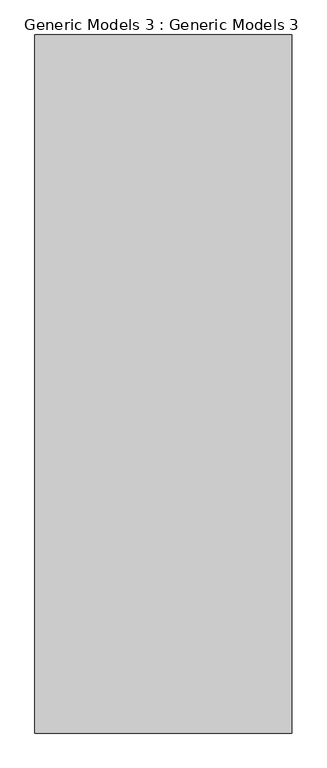
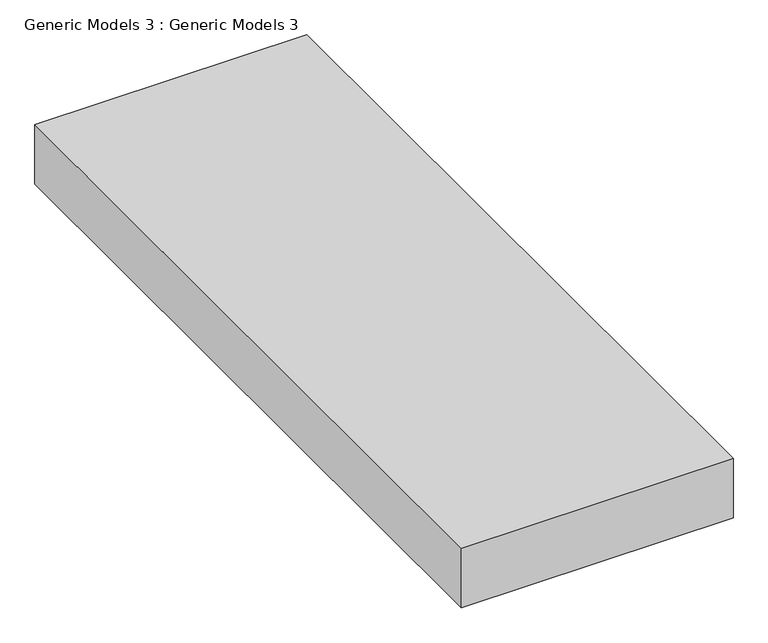
"""IFC4 building model written with IfcOpenShell, lengths in millimetres: proxy geometry, Generic Models 3 : Generic Models 3."""

from ifc_helpers import new_model, si_unit, frame, origin, place, context, project, spatial, polyline, outline, extrude, source, transform, mapped, element, save


def generic_models_3_generic_models_3_8d4ae4f9(model_context):
    return source(origin(), model_context, "Body", "SweptSolid", [
        extrude(outline(polyline([(-18499.9023139, -8772.8322282), (-17842.4229687, -8772.8322282), (-17842.4229687, -10561.1015118), (-18499.9023139, -10561.1015118), (-18499.9023139, -8772.8322282)])), frame((0.0, 0.0, 5516.2672692), z_axis=(0.0, 0.0, 1.0), x_axis=(1.0, 0.0, 0.0)), (0.0, 0.0, 1.0), 152.4),
    ])


if __name__ == "__main__":
    model = new_model("IFC4")
    model_context = context("Model", 3, world=origin())
    ifc_project = project(units=[si_unit("LENGTHUNIT", "METRE", prefix="MILLI")], contexts=[model_context])
    site = spatial("IfcSite", under=ifc_project)
    building = spatial("IfcBuilding", under=site)
    placement = place(None, origin())
    generic_models_3_generic_models_3_shape = generic_models_3_generic_models_3_8d4ae4f9(model_context)
    element("IfcBuildingElementProxy", 1, Name="Generic Models 3 : Generic Models 3", ObjectType="Generic Models 3 : Generic Models 3", at=placement, inside=building, context=model_context, shape_type="MappedRepresentation", body=[
        mapped(generic_models_3_generic_models_3_shape, transform((0.0, 0.0, 0.0), x_axis=(1.0, 0.0, 0.0), y_axis=(0.0, 1.0, 0.0), z_axis=(0.0, 0.0, 1.0))),
    ])
    save(model, "model.ifc")
